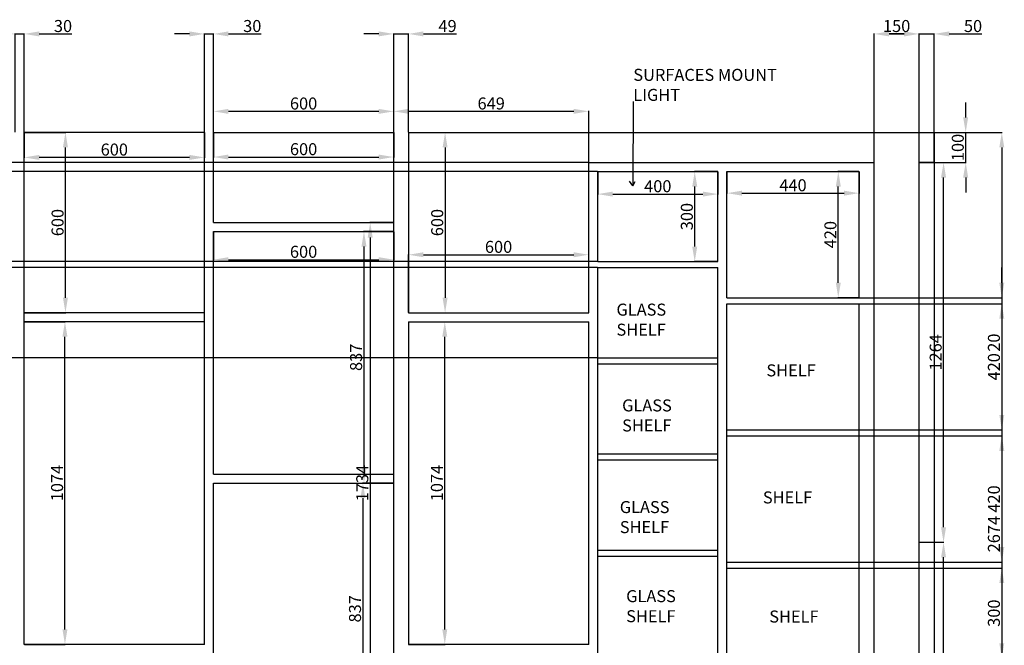
# Model space of a CAD drawing. Units: millimetres. Extents: x -2182 to 7969, y 257 to 4097.
# Tile 5 of 5: x 4692 to 7969, y 1457 to 3539. Entities that reach past the tile are written whole.
import ezdxf

# ---------------------------------------------------------------- set-up
doc = ezdxf.new("R2010")
doc.units = ezdxf.units.MM
for name, color, linetype, lineweight in [('A-ANNO-DIMS', 2, 'Continuous', 18), ('A-ANNO-TEXT', 3, 'Continuous', 18), ('A-ELEV', 7, 'Continuous', 25)]:
    doc.layers.add(name, color=color, linetype=linetype, lineweight=lineweight)
doc.styles.get("Standard").update_dxf_attribs({"font": 'arial.ttf'})
doc.dimstyles.new('ISO-25', dxfattribs={"dimtxt": 40, "dimasz": 50, "dimexe": 1.25, "dimexo": 0.625, "dimtad": 1, "dimtxsty": 'Standard', "dimcen": 2.5, "dimadec": 0, "dimazin": 0, "dimtfac": 1, "dimtmove": 0, "dimatfit": 3, "dimfxl": 1, "dimarcsym": 0})

# ---------------------------------------------------------------- blocks, each defined once
blk = doc.blocks.new('*D53')
at = {"layer": 'A-ANNO-DIMS', "color": 0, "lineweight": -2, "transparency": 16777216}
for p, q in [((7686.6, 1800), (7768.3, 1800)), ((7767.1, 650), (7767.1, 1750)), ((7536.6, 600), (7768.3, 600))]:
    blk.add_line(p, q, dxfattribs=at)
at = {"layer": 'A-ANNO-DIMS', "color": 0, "transparency": 16777216}
for points in [[(7758.7, 1750), (7775.4, 1750), (7767.1, 1800)], [(7758.7, 650), (7775.4, 650), (7767.1, 600)]]:
    blk.add_solid(points, dxfattribs=at)
at = {"layer": 'Defpoints', "color": 0, "transparency": 16777216}
for p in [(7685.9, 1800), (7767.1, 1800), (7535.9, 600)]:
    blk.add_point(p, dxfattribs=at)
at = {"layer": 'A-ANNO-DIMS', "color": 0, "transparency": 16777216, "insert": (7746, 1200), "char_height": 40, "attachment_point": 5, "rotation": 90}
blk.add_mtext('1200', dxfattribs=at)
blk = doc.blocks.new('*D50')
at = {"layer": 'A-ANNO-DIMS', "color": 0, "lineweight": -2, "transparency": 16777216}
for p, q in [((7686.6, 3064), (7768.3, 3064)), ((7767.1, 1850), (7767.1, 3014)), ((7686.6, 1800), (7768.3, 1800))]:
    blk.add_line(p, q, dxfattribs=at)
at = {"layer": 'A-ANNO-DIMS', "color": 0, "transparency": 16777216}
for points in [[(7758.7, 3014), (7775.4, 3014), (7767.1, 3064)], [(7758.7, 1850), (7775.4, 1850), (7767.1, 1800)]]:
    blk.add_solid(points, dxfattribs=at)
at = {"layer": 'Defpoints', "color": 0, "transparency": 16777216}
for p in [(7685.9, 3064), (7767.1, 3064), (7685.9, 1800)]:
    blk.add_point(p, dxfattribs=at)
at = {"layer": 'A-ANNO-DIMS', "color": 0, "transparency": 16777216, "insert": (7746, 2432), "char_height": 40, "attachment_point": 5, "rotation": 90}
blk.add_mtext('1264', dxfattribs=at)
blk = doc.blocks.new('*D51')
at = {"layer": 'A-ANNO-DIMS', "color": 0, "lineweight": -2, "transparency": 16777216}
for p, q in [((7840.7, 3214), (7840.7, 3264)), ((7736.6, 3164), (7841.9, 3164)), ((7840.7, 3064), (7840.7, 3164)), ((7737.8, 3064), (7841.9, 3064)), ((7840.7, 3014), (7840.7, 2964))]:
    blk.add_line(p, q, dxfattribs=at)
at = {"layer": 'A-ANNO-DIMS', "color": 0, "transparency": 16777216}
for points in [[(7832.3, 3214), (7849, 3214), (7840.7, 3164)], [(7832.3, 3014), (7849, 3014), (7840.7, 3064)]]:
    blk.add_solid(points, dxfattribs=at)
at = {"layer": 'Defpoints', "color": 0, "transparency": 16777216}
for p in [(7735.9, 3164), (7840.7, 3164), (7737.2, 3064)]:
    blk.add_point(p, dxfattribs=at)
at = {"layer": 'A-ANNO-DIMS', "color": 0, "transparency": 16777216, "insert": (7819.6, 3114), "char_height": 40, "attachment_point": 5, "rotation": 90}
blk.add_mtext('100', dxfattribs=at)
blk = doc.blocks.new('*D37')
at = {"layer": 'A-ANNO-DIMS', "color": 0, "lineweight": -2, "transparency": 16777216}
for p, q in [((5985.9, 2564.6), (5985.9, 2758.2)), ((6035.9, 2757), (6535.9, 2757)), ((6585.9, 2564.6), (6585.9, 2758.2))]:
    blk.add_line(p, q, dxfattribs=at)
at = {"layer": 'A-ANNO-DIMS', "color": 0, "transparency": 16777216}
for points in [[(6035.9, 2765.3), (6035.9, 2748.6), (5985.9, 2757)], [(6535.9, 2765.3), (6535.9, 2748.6), (6585.9, 2757)]]:
    blk.add_solid(points, dxfattribs=at)
at = {"layer": 'Defpoints', "color": 0, "transparency": 16777216}
for p in [(6585.9, 2757), (5985.9, 2564), (6585.9, 2564)]:
    blk.add_point(p, dxfattribs=at)
at = {"layer": 'A-ANNO-DIMS', "color": 0, "transparency": 16777216, "insert": (6285.9, 2778), "char_height": 40, "attachment_point": 5}
blk.add_mtext('600', dxfattribs=at)
blk = doc.blocks.new('*D38')
at = {"layer": 'A-ANNO-DIMS', "color": 0, "lineweight": -2, "transparency": 16777216}
for p, q in [((5986.6, 3164), (6109.1, 3164)), ((6107.9, 3114), (6107.9, 2614)), ((5986.6, 2564), (6109.1, 2564))]:
    blk.add_line(p, q, dxfattribs=at)
at = {"layer": 'A-ANNO-DIMS', "color": 0, "transparency": 16777216}
for points in [[(6099.5, 3114), (6116.2, 3114), (6107.9, 3164)], [(6099.5, 2614), (6116.2, 2614), (6107.9, 2564)]]:
    blk.add_solid(points, dxfattribs=at)
at = {"layer": 'Defpoints', "color": 0, "transparency": 16777216}
for p in [(5985.9, 3164), (5985.9, 2564), (6107.9, 2564)]:
    blk.add_point(p, dxfattribs=at)
at = {"layer": 'A-ANNO-DIMS', "color": 0, "transparency": 16777216, "insert": (6086.8, 2864), "char_height": 40, "attachment_point": 5, "rotation": 90}
blk.add_mtext('600', dxfattribs=at)
blk = doc.blocks.new('*D31')
at = {"layer": 'A-ANNO-DIMS', "color": 0, "lineweight": -2, "transparency": 16777216}
for p, q in [((5986.6, 2534), (6108.1, 2534)), ((6106.9, 1510), (6106.9, 2484)), ((5986.6, 1460), (6108.1, 1460))]:
    blk.add_line(p, q, dxfattribs=at)
at = {"layer": 'A-ANNO-DIMS', "color": 0, "transparency": 16777216}
for points in [[(6098.5, 2484), (6115.2, 2484), (6106.9, 2534)], [(6098.5, 1510), (6115.2, 1510), (6106.9, 1460)]]:
    blk.add_solid(points, dxfattribs=at)
at = {"layer": 'Defpoints', "color": 0, "transparency": 16777216}
for p in [(5985.9, 2534), (6106.9, 2534), (5985.9, 1460)]:
    blk.add_point(p, dxfattribs=at)
at = {"layer": 'A-ANNO-DIMS', "color": 0, "transparency": 16777216, "insert": (6085.8, 1997), "char_height": 40, "attachment_point": 5, "rotation": 90}
blk.add_mtext('1074', dxfattribs=at)
blk = doc.blocks.new('*D39')
at = {"layer": 'A-ANNO-DIMS', "color": 0, "lineweight": -2, "transparency": 16777216}
for p, q in [((5936.9, 3164.6), (5936.9, 3235.5)), ((6535.9, 3234.3), (5986.9, 3234.3)), ((6585.9, 3164.6), (6585.9, 3235.5))]:
    blk.add_line(p, q, dxfattribs=at)
at = {"layer": 'A-ANNO-DIMS', "color": 0, "transparency": 16777216}
for points in [[(5986.9, 3242.6), (5986.9, 3225.9), (5936.9, 3234.3)], [(6535.9, 3242.6), (6535.9, 3225.9), (6585.9, 3234.3)]]:
    blk.add_solid(points, dxfattribs=at)
at = {"layer": 'Defpoints', "color": 0, "transparency": 16777216}
for p in [(5936.9, 3234.3), (5936.9, 3164), (6585.9, 3164)]:
    blk.add_point(p, dxfattribs=at)
at = {"layer": 'A-ANNO-DIMS', "color": 0, "transparency": 16777216, "insert": (6261.4, 3255.3), "char_height": 40, "attachment_point": 5}
blk.add_mtext('649', dxfattribs=at)
blk = doc.blocks.new('*D40')
at = {"layer": 'A-ANNO-DIMS', "color": 0, "lineweight": -2, "transparency": 16777216}
for p, q in [((5936.3, 2864), (5857.3, 2864)), ((5858.6, 2814), (5858.6, 1180)), ((5936.3, 1130), (5857.3, 1130))]:
    blk.add_line(p, q, dxfattribs=at)
at = {"layer": 'A-ANNO-DIMS', "color": 0, "transparency": 16777216}
for points in [[(5850.2, 2814), (5866.9, 2814), (5858.6, 2864)], [(5850.2, 1180), (5866.9, 1180), (5858.6, 1130)]]:
    blk.add_solid(points, dxfattribs=at)
at = {"layer": 'Defpoints', "color": 0, "transparency": 16777216}
for p in [(5936.9, 2864), (5858.6, 1130), (5936.9, 1130)]:
    blk.add_point(p, dxfattribs=at)
at = {"layer": 'A-ANNO-DIMS', "color": 0, "transparency": 16777216, "insert": (5837.5, 1997), "char_height": 40, "attachment_point": 5, "rotation": 90}
blk.add_mtext('1734', dxfattribs=at)
blk = doc.blocks.new('*D41')
at = {"layer": 'A-ANNO-DIMS', "color": 0, "lineweight": -2, "transparency": 16777216}
for p, q in [((5336.9, 2833.4), (5336.9, 2739.3)), ((5936.9, 2833.4), (5936.9, 2739.3)), ((5386.9, 2740.5), (5886.9, 2740.5))]:
    blk.add_line(p, q, dxfattribs=at)
at = {"layer": 'A-ANNO-DIMS', "color": 0, "transparency": 16777216}
for points in [[(5386.9, 2748.8), (5386.9, 2732.2), (5336.9, 2740.5)], [(5886.9, 2748.8), (5886.9, 2732.2), (5936.9, 2740.5)]]:
    blk.add_solid(points, dxfattribs=at)
at = {"layer": 'Defpoints', "color": 0, "transparency": 16777216}
for p in [(5336.9, 2834), (5936.9, 2834), (5936.9, 2740.5)]:
    blk.add_point(p, dxfattribs=at)
at = {"layer": 'A-ANNO-DIMS', "color": 0, "transparency": 16777216, "insert": (5636.9, 2761.6), "char_height": 40, "attachment_point": 5}
blk.add_mtext('600', dxfattribs=at)
blk = doc.blocks.new('*D42')
at = {"layer": 'A-ANNO-DIMS', "color": 0, "lineweight": -2, "transparency": 16777216}
for p, q in [((5936.3, 2834), (5836.7, 2834)), ((5837.9, 2784), (5837.9, 2047)), ((5936.3, 1997), (5836.7, 1997))]:
    blk.add_line(p, q, dxfattribs=at)
at = {"layer": 'A-ANNO-DIMS', "color": 0, "transparency": 16777216}
for points in [[(5829.6, 2784), (5846.3, 2784), (5837.9, 2834)], [(5829.6, 2047), (5846.3, 2047), (5837.9, 1997)]]:
    blk.add_solid(points, dxfattribs=at)
at = {"layer": 'Defpoints', "color": 0, "transparency": 16777216}
for p in [(5936.9, 2834), (5837.9, 1997), (5936.9, 1997)]:
    blk.add_point(p, dxfattribs=at)
at = {"layer": 'A-ANNO-DIMS', "color": 0, "transparency": 16777216, "insert": (5816.9, 2415.5), "char_height": 40, "attachment_point": 5, "rotation": 90}
blk.add_mtext('837', dxfattribs=at)
blk = doc.blocks.new('*D43')
at = {"layer": 'A-ANNO-DIMS', "color": 0, "lineweight": -2, "transparency": 16777216}
for p, q in [((5336.9, 3163.4), (5336.9, 3080.9)), ((5936.9, 3163.4), (5936.9, 3080.9)), ((5386.9, 3082.2), (5886.9, 3082.2))]:
    blk.add_line(p, q, dxfattribs=at)
at = {"layer": 'A-ANNO-DIMS', "color": 0, "transparency": 16777216}
for points in [[(5386.9, 3090.5), (5386.9, 3073.9), (5336.9, 3082.2)], [(5886.9, 3090.5), (5886.9, 3073.9), (5936.9, 3082.2)]]:
    blk.add_solid(points, dxfattribs=at)
at = {"layer": 'Defpoints', "color": 0, "transparency": 16777216}
for p in [(5336.9, 3164), (5936.9, 3164), (5936.9, 3082.2)]:
    blk.add_point(p, dxfattribs=at)
at = {"layer": 'A-ANNO-DIMS', "color": 0, "transparency": 16777216, "insert": (5636.9, 3103.2), "char_height": 40, "attachment_point": 5}
blk.add_mtext('600', dxfattribs=at)
blk = doc.blocks.new('*D33')
at = {"layer": 'A-ANNO-DIMS', "color": 0, "lineweight": -2, "transparency": 16777216}
for p, q in [((5936.3, 1997), (5833.1, 1997)), ((5834.4, 1947), (5834.4, 1210)), ((5936.3, 1160), (5833.1, 1160))]:
    blk.add_line(p, q, dxfattribs=at)
at = {"layer": 'A-ANNO-DIMS', "color": 0, "transparency": 16777216}
for points in [[(5826, 1947), (5842.7, 1947), (5834.4, 1997)], [(5826, 1210), (5842.7, 1210), (5834.4, 1160)]]:
    blk.add_solid(points, dxfattribs=at)
at = {"layer": 'Defpoints', "color": 0, "transparency": 16777216}
for p in [(5936.9, 1997), (5834.4, 1160), (5936.9, 1160)]:
    blk.add_point(p, dxfattribs=at)
at = {"layer": 'A-ANNO-DIMS', "color": 0, "transparency": 16777216, "insert": (5813.3, 1578.5), "char_height": 40, "attachment_point": 5, "rotation": 90}
blk.add_mtext('837', dxfattribs=at)
blk = doc.blocks.new('*D45')
at = {"layer": 'A-ANNO-DIMS', "color": 0, "lineweight": -2, "transparency": 16777216}
for p, q in [((5336.9, 3164.6), (5336.9, 3235.4)), ((5886.9, 3234.2), (5386.9, 3234.2)), ((5936.9, 3164.6), (5936.9, 3235.4))]:
    blk.add_line(p, q, dxfattribs=at)
at = {"layer": 'A-ANNO-DIMS', "color": 0, "transparency": 16777216}
for points in [[(5386.9, 3242.5), (5386.9, 3225.8), (5336.9, 3234.2)], [(5886.9, 3242.5), (5886.9, 3225.8), (5936.9, 3234.2)]]:
    blk.add_solid(points, dxfattribs=at)
at = {"layer": 'Defpoints', "color": 0, "transparency": 16777216}
for p in [(5336.9, 3234.2), (5336.9, 3164), (5936.9, 3164)]:
    blk.add_point(p, dxfattribs=at)
at = {"layer": 'A-ANNO-DIMS', "color": 0, "transparency": 16777216, "insert": (5636.9, 3255.2), "char_height": 40, "attachment_point": 5}
blk.add_mtext('600', dxfattribs=at)
blk = doc.blocks.new('*D48')
at = {"layer": 'A-ANNO-DIMS', "color": 0, "lineweight": -2, "transparency": 16777216}
for p, q in [((4707.6, 2534), (4843.8, 2534)), ((4842.6, 1510), (4842.6, 2484)), ((4707.6, 1460), (4843.8, 1460))]:
    blk.add_line(p, q, dxfattribs=at)
at = {"layer": 'A-ANNO-DIMS', "color": 0, "transparency": 16777216}
for points in [[(4834.2, 2484), (4850.9, 2484), (4842.6, 2534)], [(4834.2, 1510), (4850.9, 1510), (4842.6, 1460)]]:
    blk.add_solid(points, dxfattribs=at)
at = {"layer": 'Defpoints', "color": 0, "transparency": 16777216}
for p in [(4706.9, 2534), (4842.6, 2534), (4706.9, 1460)]:
    blk.add_point(p, dxfattribs=at)
at = {"layer": 'A-ANNO-DIMS', "color": 0, "transparency": 16777216, "insert": (4821.5, 1997), "char_height": 40, "attachment_point": 5, "rotation": 90}
blk.add_mtext('1074', dxfattribs=at)
blk = doc.blocks.new('*D49')
at = {"layer": 'A-ANNO-DIMS', "color": 0, "lineweight": -2, "transparency": 16777216}
for p, q in [((4707.6, 3164), (4845.5, 3164)), ((4844.2, 2614), (4844.2, 3114)), ((4707.6, 2564), (4845.5, 2564))]:
    blk.add_line(p, q, dxfattribs=at)
at = {"layer": 'A-ANNO-DIMS', "color": 0, "transparency": 16777216}
for points in [[(4835.9, 3114), (4852.6, 3114), (4844.2, 3164)], [(4835.9, 2614), (4852.6, 2614), (4844.2, 2564)]]:
    blk.add_solid(points, dxfattribs=at)
at = {"layer": 'Defpoints', "color": 0, "transparency": 16777216}
for p in [(4706.9, 3164), (4844.2, 3164), (4706.9, 2564)]:
    blk.add_point(p, dxfattribs=at)
at = {"layer": 'A-ANNO-DIMS', "color": 0, "transparency": 16777216, "insert": (4823.2, 2864), "char_height": 40, "attachment_point": 5, "rotation": 90}
blk.add_mtext('600', dxfattribs=at)
blk = doc.blocks.new('*D46')
at = {"layer": 'A-ANNO-DIMS', "color": 0, "lineweight": -2, "transparency": 16777216}
for p, q in [((4706.9, 3163.4), (4706.9, 3079.6)), ((5306.9, 3163.4), (5306.9, 3079.6)), ((5256.9, 3080.9), (4756.9, 3080.9))]:
    blk.add_line(p, q, dxfattribs=at)
at = {"layer": 'A-ANNO-DIMS', "color": 0, "transparency": 16777216}
for points in [[(4756.9, 3089.2), (4756.9, 3072.5), (4706.9, 3080.9)], [(5256.9, 3089.2), (5256.9, 3072.5), (5306.9, 3080.9)]]:
    blk.add_solid(points, dxfattribs=at)
at = {"layer": 'Defpoints', "color": 0, "transparency": 16777216}
for p in [(4706.9, 3164), (5306.9, 3164), (4706.9, 3080.9)]:
    blk.add_point(p, dxfattribs=at)
at = {"layer": 'A-ANNO-DIMS', "color": 0, "transparency": 16777216, "insert": (5006.9, 3101.9), "char_height": 40, "attachment_point": 5}
blk.add_mtext('600', dxfattribs=at)
blk = doc.blocks.new('*D57')
at = {"layer": 'A-ANNO-DIMS', "color": 0, "lineweight": -2, "transparency": 16777216}
for p, q in [((7015.3, 3034), (6937.6, 3034)), ((6938.8, 2784), (6938.8, 2984)), ((7015.3, 2734), (6937.6, 2734))]:
    blk.add_line(p, q, dxfattribs=at)
at = {"layer": 'A-ANNO-DIMS', "color": 0, "transparency": 16777216}
for points in [[(6930.5, 2984), (6947.2, 2984), (6938.8, 3034)], [(6930.5, 2784), (6947.2, 2784), (6938.8, 2734)]]:
    blk.add_solid(points, dxfattribs=at)
at = {"layer": 'Defpoints', "color": 0, "transparency": 16777216}
for p in [(6938.8, 3034), (7015.9, 3034), (7015.9, 2734)]:
    blk.add_point(p, dxfattribs=at)
at = {"layer": 'A-ANNO-DIMS', "color": 0, "transparency": 16777216, "insert": (6917.8, 2884), "char_height": 40, "attachment_point": 5, "rotation": 90}
blk.add_mtext('300', dxfattribs=at)
blk = doc.blocks.new('*D58')
at = {"layer": 'A-ANNO-DIMS', "color": 0, "lineweight": -2, "transparency": 16777216}
for p, q in [((6615.9, 3033.4), (6615.9, 2957.6)), ((7015.9, 3033.4), (7015.9, 2957.6)), ((6665.9, 2958.8), (6965.9, 2958.8))]:
    blk.add_line(p, q, dxfattribs=at)
at = {"layer": 'A-ANNO-DIMS', "color": 0, "transparency": 16777216}
for points in [[(6665.9, 2967.2), (6665.9, 2950.5), (6615.9, 2958.8)], [(6965.9, 2967.2), (6965.9, 2950.5), (7015.9, 2958.8)]]:
    blk.add_solid(points, dxfattribs=at)
at = {"layer": 'Defpoints', "color": 0, "transparency": 16777216}
for p in [(6615.9, 3034), (7015.9, 3034), (7015.9, 2958.8)]:
    blk.add_point(p, dxfattribs=at)
at = {"layer": 'A-ANNO-DIMS', "color": 0, "transparency": 16777216, "insert": (6815.9, 2979.9), "char_height": 40, "attachment_point": 5}
blk.add_mtext('400', dxfattribs=at)
blk = doc.blocks.new('*D59')
at = {"layer": 'A-ANNO-DIMS', "color": 0, "lineweight": -2, "transparency": 16777216}
for p, q in [((7045.9, 3033.4), (7045.9, 2960.7)), ((7485.9, 3033.4), (7485.9, 2960.7)), ((7095.9, 2961.9), (7435.9, 2961.9))]:
    blk.add_line(p, q, dxfattribs=at)
at = {"layer": 'A-ANNO-DIMS', "color": 0, "transparency": 16777216}
for points in [[(7095.9, 2970.3), (7095.9, 2953.6), (7045.9, 2961.9)], [(7435.9, 2970.3), (7435.9, 2953.6), (7485.9, 2961.9)]]:
    blk.add_solid(points, dxfattribs=at)
at = {"layer": 'Defpoints', "color": 0, "transparency": 16777216}
for p in [(7045.9, 3034), (7485.9, 3034), (7485.9, 2961.9)]:
    blk.add_point(p, dxfattribs=at)
at = {"layer": 'A-ANNO-DIMS', "color": 0, "transparency": 16777216, "insert": (7265.9, 2983), "char_height": 40, "attachment_point": 5}
blk.add_mtext('440', dxfattribs=at)
blk = doc.blocks.new('*D60')
at = {"layer": 'A-ANNO-DIMS', "color": 0, "lineweight": -2, "transparency": 16777216}
for p, q in [((7485.3, 3034), (7415.5, 3034)), ((7416.7, 2664), (7416.7, 2984)), ((7485.3, 2614), (7415.5, 2614))]:
    blk.add_line(p, q, dxfattribs=at)
at = {"layer": 'A-ANNO-DIMS', "color": 0, "transparency": 16777216}
for points in [[(7408.4, 2984), (7425, 2984), (7416.7, 3034)], [(7408.4, 2664), (7425, 2664), (7416.7, 2614)]]:
    blk.add_solid(points, dxfattribs=at)
at = {"layer": 'Defpoints', "color": 0, "transparency": 16777216}
for p in [(7416.7, 3034), (7485.9, 3034), (7485.9, 2614)]:
    blk.add_point(p, dxfattribs=at)
at = {"layer": 'A-ANNO-DIMS', "color": 0, "transparency": 16777216, "insert": (7395.7, 2824), "char_height": 40, "attachment_point": 5, "rotation": 90}
blk.add_mtext('420', dxfattribs=at)
blk = doc.blocks.new('*D77')
at = {"layer": 'A-ANNO-DIMS', "color": 0, "lineweight": -2, "transparency": 16777216}
for p, q in [((7735.9, 3063.4), (7735.9, 263.7)), ((3426.9, 489.4), (3426.9, 263.7)), ((3476.9, 265), (7685.9, 265))]:
    blk.add_line(p, q, dxfattribs=at)
at = {"layer": 'A-ANNO-DIMS', "color": 0, "transparency": 16777216}
for points in [[(3476.9, 273.3), (3476.9, 256.7), (3426.9, 265)], [(7685.9, 273.3), (7685.9, 256.7), (7735.9, 265)]]:
    blk.add_solid(points, dxfattribs=at)
at = {"layer": 'Defpoints', "color": 0, "transparency": 16777216}
for p in [(7735.9, 3064), (3426.9, 490), (7735.9, 265)]:
    blk.add_point(p, dxfattribs=at)
at = {"layer": 'A-ANNO-DIMS', "color": 0, "transparency": 16777216, "insert": (5581.4, 286.1), "char_height": 40, "attachment_point": 5}
blk.add_mtext('4309', dxfattribs=at)
blk = doc.blocks.new('*D79')
at = {"layer": 'A-ANNO-DIMS', "color": 0, "lineweight": -2, "transparency": 16777216}
for p, q in [((7736.6, 3164), (7962.2, 3164)), ((7960.9, 3114), (7960.9, 540)), ((3427.6, 490), (7962.2, 490))]:
    blk.add_line(p, q, dxfattribs=at)
at = {"layer": 'A-ANNO-DIMS', "color": 0, "transparency": 16777216}
for points in [[(7952.6, 3114), (7969.3, 3114), (7960.9, 3164)], [(7952.6, 540), (7969.3, 540), (7960.9, 490)]]:
    blk.add_solid(points, dxfattribs=at)
at = {"layer": 'Defpoints', "color": 0, "transparency": 16777216}
for p in [(7735.9, 3164), (3426.9, 490), (7960.9, 490)]:
    blk.add_point(p, dxfattribs=at)
at = {"layer": 'A-ANNO-DIMS', "color": 0, "transparency": 16777216, "insert": (7939.9, 1827), "char_height": 40, "attachment_point": 5, "rotation": 90}
blk.add_mtext('2674', dxfattribs=at)
blk = doc.blocks.new('*D82')
at = {"layer": 'A-ANNO-DIMS', "color": 0, "lineweight": -2, "transparency": 16777216}
for p, q in [((4626.9, 3492), (4576.9, 3492)), ((4676.9, 3164.6), (4676.9, 3493.3)), ((4676.9, 3492), (4706.9, 3492)), ((4706.9, 3164.6), (4706.9, 3493.3)), ((4756.9, 3492), (4865.3, 3492))]:
    blk.add_line(p, q, dxfattribs=at)
at = {"layer": 'A-ANNO-DIMS', "color": 0, "transparency": 16777216}
for points in [[(4626.9, 3500.4), (4626.9, 3483.7), (4676.9, 3492)], [(4756.9, 3500.4), (4756.9, 3483.7), (4706.9, 3492)]]:
    blk.add_solid(points, dxfattribs=at)
at = {"layer": 'Defpoints', "color": 0, "transparency": 16777216}
for p in [(4706.9, 3492), (4676.9, 3164), (4706.9, 3164)]:
    blk.add_point(p, dxfattribs=at)
at = {"layer": 'A-ANNO-DIMS', "color": 0, "transparency": 16777216, "insert": (4836.1, 3513.1), "char_height": 40, "attachment_point": 5}
blk.add_mtext('30', dxfattribs=at)
blk = doc.blocks.new('*D83')
at = {"layer": 'A-ANNO-DIMS', "color": 0, "lineweight": -2, "transparency": 16777216}
for p, q in [((5256.9, 3492), (5206.9, 3492)), ((5306.9, 3164.6), (5306.9, 3493.3)), ((5306.9, 3492), (5336.9, 3492)), ((5336.9, 3164.6), (5336.9, 3493.3)), ((5386.9, 3492), (5495.3, 3492))]:
    blk.add_line(p, q, dxfattribs=at)
at = {"layer": 'A-ANNO-DIMS', "color": 0, "transparency": 16777216}
for points in [[(5256.9, 3500.4), (5256.9, 3483.7), (5306.9, 3492)], [(5386.9, 3500.4), (5386.9, 3483.7), (5336.9, 3492)]]:
    blk.add_solid(points, dxfattribs=at)
at = {"layer": 'Defpoints', "color": 0, "transparency": 16777216}
for p in [(5336.9, 3492), (5306.9, 3164), (5336.9, 3164)]:
    blk.add_point(p, dxfattribs=at)
at = {"layer": 'A-ANNO-DIMS', "color": 0, "transparency": 16777216, "insert": (5466.1, 3513.1), "char_height": 40, "attachment_point": 5}
blk.add_mtext('30', dxfattribs=at)
blk = doc.blocks.new('*D84')
at = {"layer": 'A-ANNO-DIMS', "color": 0, "lineweight": -2, "transparency": 16777216}
for p, q in [((5886.9, 3492), (5836.9, 3492)), ((5936.9, 3164.6), (5936.9, 3493.3)), ((5936.9, 3492), (5985.9, 3492)), ((5985.9, 3164.6), (5985.9, 3493.3)), ((6035.9, 3492), (6146.2, 3492))]:
    blk.add_line(p, q, dxfattribs=at)
at = {"layer": 'A-ANNO-DIMS', "color": 0, "transparency": 16777216}
for points in [[(5886.9, 3500.4), (5886.9, 3483.7), (5936.9, 3492)], [(6035.9, 3500.4), (6035.9, 3483.7), (5985.9, 3492)]]:
    blk.add_solid(points, dxfattribs=at)
at = {"layer": 'Defpoints', "color": 0, "transparency": 16777216}
for p in [(5985.9, 3492), (5936.9, 3164), (5985.9, 3164)]:
    blk.add_point(p, dxfattribs=at)
at = {"layer": 'A-ANNO-DIMS', "color": 0, "transparency": 16777216, "insert": (6116.1, 3513.1), "char_height": 40, "attachment_point": 5}
blk.add_mtext('49', dxfattribs=at)
blk = doc.blocks.new('*D88')
at = {"layer": 'A-ANNO-DIMS', "color": 0, "lineweight": -2, "transparency": 16777216}
for p, q in [((7535.9, 3064.6), (7535.9, 3493.3)), ((7585.9, 3492), (7635.9, 3492)), ((7685.9, 3064.6), (7685.9, 3493.3))]:
    blk.add_line(p, q, dxfattribs=at)
at = {"layer": 'A-ANNO-DIMS', "color": 0, "transparency": 16777216}
for points in [[(7585.9, 3500.4), (7585.9, 3483.7), (7535.9, 3492)], [(7635.9, 3500.4), (7635.9, 3483.7), (7685.9, 3492)]]:
    blk.add_solid(points, dxfattribs=at)
at = {"layer": 'Defpoints', "color": 0, "transparency": 16777216}
for p in [(7685.9, 3492), (7535.9, 3064), (7685.9, 3064)]:
    blk.add_point(p, dxfattribs=at)
at = {"layer": 'A-ANNO-DIMS', "color": 0, "transparency": 16777216, "insert": (7610.9, 3513.1), "char_height": 40, "attachment_point": 5}
blk.add_mtext('150', dxfattribs=at)
blk = doc.blocks.new('*D89')
at = {"layer": 'A-ANNO-DIMS', "color": 0, "lineweight": -2, "transparency": 16777216}
for p, q in [((7635.9, 3492), (7585.9, 3492)), ((7685.9, 3064.6), (7685.9, 3493.3)), ((7685.9, 3492), (7735.9, 3492)), ((7735.9, 3064.6), (7735.9, 3493.3)), ((7785.9, 3492), (7894.4, 3492))]:
    blk.add_line(p, q, dxfattribs=at)
at = {"layer": 'A-ANNO-DIMS', "color": 0, "transparency": 16777216}
for points in [[(7635.9, 3500.4), (7635.9, 3483.7), (7685.9, 3492)], [(7785.9, 3500.4), (7785.9, 3483.7), (7735.9, 3492)]]:
    blk.add_solid(points, dxfattribs=at)
at = {"layer": 'Defpoints', "color": 0, "transparency": 16777216}
for p in [(7735.9, 3492), (7685.9, 3064), (7735.9, 3064)]:
    blk.add_point(p, dxfattribs=at)
at = {"layer": 'A-ANNO-DIMS', "color": 0, "transparency": 16777216, "insert": (7865.2, 3513.1), "char_height": 40, "attachment_point": 5}
blk.add_mtext('50', dxfattribs=at)
blk = doc.blocks.new('*D92')
at = {"layer": 'A-ANNO-DIMS', "color": 0, "lineweight": -2, "transparency": 16777216}
for p, q in [((3201.9, 3114), (3201.9, 3164)), ((6585.3, 3064), (3200.7, 3064)), ((3201.9, 3064), (3201.9, 3034)), ((6615.3, 3034), (3200.7, 3034)), ((3201.9, 2984), (3201.9, 2875.6))]:
    blk.add_line(p, q, dxfattribs=at)
at = {"layer": 'A-ANNO-DIMS', "color": 0, "transparency": 16777216}
for points in [[(3193.6, 3114), (3210.3, 3114), (3201.9, 3064)], [(3193.6, 2984), (3210.3, 2984), (3201.9, 3034)]]:
    blk.add_solid(points, dxfattribs=at)
at = {"layer": 'Defpoints', "color": 0, "transparency": 16777216}
for p in [(6585.9, 3064), (3201.9, 3034), (6615.9, 3034)]:
    blk.add_point(p, dxfattribs=at)
at = {"layer": 'A-ANNO-DIMS', "color": 0, "transparency": 16777216, "insert": (3180.9, 2904.8), "char_height": 40, "attachment_point": 5, "rotation": 90}
blk.add_mtext('30', dxfattribs=at)
blk = doc.blocks.new('*D93')
at = {"layer": 'A-ANNO-DIMS', "color": 0, "lineweight": -2, "transparency": 16777216}
for p, q in [((3201.9, 2784), (3201.9, 2834)), ((6615.3, 2734), (3200.7, 2734)), ((3201.9, 2734), (3201.9, 2714)), ((6615.3, 2714), (3200.7, 2714)), ((3201.9, 2664), (3201.9, 2554.9))]:
    blk.add_line(p, q, dxfattribs=at)
at = {"layer": 'A-ANNO-DIMS', "color": 0, "transparency": 16777216}
for points in [[(3193.6, 2784), (3210.3, 2784), (3201.9, 2734)], [(3193.6, 2664), (3210.3, 2664), (3201.9, 2714)]]:
    blk.add_solid(points, dxfattribs=at)
at = {"layer": 'Defpoints', "color": 0, "transparency": 16777216}
for p in [(6615.9, 2734), (3201.9, 2714), (6615.9, 2714)]:
    blk.add_point(p, dxfattribs=at)
at = {"layer": 'A-ANNO-DIMS', "color": 0, "transparency": 16777216, "insert": (3180.9, 2584.4), "char_height": 40, "attachment_point": 5, "rotation": 90}
blk.add_mtext('20', dxfattribs=at)
blk = doc.blocks.new('*D94')
at = {"layer": 'A-ANNO-DIMS', "color": 0, "lineweight": -2, "transparency": 16777216}
for p, q in [((6615.3, 2714), (3200.7, 2714)), ((3201.9, 2664), (3201.9, 2464)), ((6615.3, 2414), (3200.7, 2414))]:
    blk.add_line(p, q, dxfattribs=at)
at = {"layer": 'A-ANNO-DIMS', "color": 0, "transparency": 16777216}
for points in [[(3193.6, 2664), (3210.3, 2664), (3201.9, 2714)], [(3193.6, 2464), (3210.3, 2464), (3201.9, 2414)]]:
    blk.add_solid(points, dxfattribs=at)
at = {"layer": 'Defpoints', "color": 0, "transparency": 16777216}
for p in [(6615.9, 2714), (3201.9, 2414), (6615.9, 2414)]:
    blk.add_point(p, dxfattribs=at)
at = {"layer": 'A-ANNO-DIMS', "color": 0, "transparency": 16777216, "insert": (3180.9, 2564), "char_height": 40, "attachment_point": 5, "rotation": 90}
blk.add_mtext('300', dxfattribs=at)
blk = doc.blocks.new('*D96')
at = {"layer": 'A-ANNO-DIMS', "color": 0, "lineweight": -2, "transparency": 16777216}
for p, q in [((7960.9, 2664), (7960.9, 2714)), ((7486.6, 2614), (7962.2, 2614)), ((7486.6, 2594), (7962.2, 2594)), ((7960.9, 2614), (7960.9, 2594)), ((7960.9, 2544), (7960.9, 2434.9))]:
    blk.add_line(p, q, dxfattribs=at)
at = {"layer": 'A-ANNO-DIMS', "color": 0, "transparency": 16777216}
for points in [[(7952.6, 2664), (7969.3, 2664), (7960.9, 2614)], [(7952.6, 2544), (7969.3, 2544), (7960.9, 2594)]]:
    blk.add_solid(points, dxfattribs=at)
at = {"layer": 'Defpoints', "color": 0, "transparency": 16777216}
for p in [(7485.9, 2614), (7485.9, 2594), (7960.9, 2594)]:
    blk.add_point(p, dxfattribs=at)
at = {"layer": 'A-ANNO-DIMS', "color": 0, "transparency": 16777216, "insert": (7939.9, 2464.4), "char_height": 40, "attachment_point": 5, "rotation": 90}
blk.add_mtext('20', dxfattribs=at)
blk = doc.blocks.new('*D97')
at = {"layer": 'A-ANNO-DIMS', "color": 0, "lineweight": -2, "transparency": 16777216}
for p, q in [((7486.6, 2594), (7962.2, 2594)), ((7960.9, 2544), (7960.9, 2224)), ((7486.6, 2174), (7962.2, 2174))]:
    blk.add_line(p, q, dxfattribs=at)
at = {"layer": 'A-ANNO-DIMS', "color": 0, "transparency": 16777216}
for points in [[(7952.6, 2544), (7969.3, 2544), (7960.9, 2594)], [(7952.6, 2224), (7969.3, 2224), (7960.9, 2174)]]:
    blk.add_solid(points, dxfattribs=at)
at = {"layer": 'Defpoints', "color": 0, "transparency": 16777216}
for p in [(7485.9, 2594), (7485.9, 2174), (7960.9, 2174)]:
    blk.add_point(p, dxfattribs=at)
at = {"layer": 'A-ANNO-DIMS', "color": 0, "transparency": 16777216, "insert": (7939.9, 2384), "char_height": 40, "attachment_point": 5, "rotation": 90}
blk.add_mtext('420', dxfattribs=at)
blk = doc.blocks.new('*D98')
at = {"layer": 'A-ANNO-DIMS', "color": 0, "lineweight": -2, "transparency": 16777216}
for p, q in [((7486.6, 2154), (7962.2, 2154)), ((7960.9, 2104), (7960.9, 1784)), ((7486.6, 1734), (7962.2, 1734))]:
    blk.add_line(p, q, dxfattribs=at)
at = {"layer": 'A-ANNO-DIMS', "color": 0, "transparency": 16777216}
for points in [[(7952.6, 2104), (7969.3, 2104), (7960.9, 2154)], [(7952.6, 1784), (7969.3, 1784), (7960.9, 1734)]]:
    blk.add_solid(points, dxfattribs=at)
at = {"layer": 'Defpoints', "color": 0, "transparency": 16777216}
for p in [(7485.9, 2154), (7485.9, 1734), (7960.9, 1734)]:
    blk.add_point(p, dxfattribs=at)
at = {"layer": 'A-ANNO-DIMS', "color": 0, "transparency": 16777216, "insert": (7939.9, 1944), "char_height": 40, "attachment_point": 5, "rotation": 90}
blk.add_mtext('420', dxfattribs=at)
blk = doc.blocks.new('*D99')
at = {"layer": 'A-ANNO-DIMS', "color": 0, "lineweight": -2, "transparency": 16777216}
for p, q in [((7486.6, 1714), (7962.2, 1714)), ((7960.9, 1664), (7960.9, 1464)), ((7486.6, 1414), (7962.2, 1414))]:
    blk.add_line(p, q, dxfattribs=at)
at = {"layer": 'A-ANNO-DIMS', "color": 0, "transparency": 16777216}
for points in [[(7952.6, 1664), (7969.3, 1664), (7960.9, 1714)], [(7952.6, 1464), (7969.3, 1464), (7960.9, 1414)]]:
    blk.add_solid(points, dxfattribs=at)
at = {"layer": 'Defpoints', "color": 0, "transparency": 16777216}
for p in [(7485.9, 1714), (7485.9, 1414), (7960.9, 1414)]:
    blk.add_point(p, dxfattribs=at)
at = {"layer": 'A-ANNO-DIMS', "color": 0, "transparency": 16777216, "insert": (7939.9, 1564), "char_height": 40, "attachment_point": 5, "rotation": 90}
blk.add_mtext('300', dxfattribs=at)

msp = doc.modelspace()

# ---------------------------------------------------------------- linework, layer by layer
at = {"layer": 'A-ELEV'}
for p, q in [((6734.4235, 3267.0268), (6733.3136, 2986.6436)), ((4706.9478, 1459.9911), (4706.9478, 3163.9911)), ((5306.9478, 3163.9911), (4706.9478, 3163.9911)), ((5306.9478, 1459.9911), (5306.9478, 3163.9911)), ((5336.9478, 2863.9911), (5336.9478, 3163.9911)), ((5336.9478, 3163.9911), (5936.9478, 3163.9911)), ((5936.9478, 1159.9911), (5936.9478, 3163.9911)), ((5985.9478, 3163.9911), (7735.9478, 3163.9911)), ((5985.9478, 3163.9911), (5985.9478, 2563.9911)), ((6585.9478, 2563.9911), (6585.9478, 3163.9911)), ((7735.9478, 3163.9911), (7735.9478, 3063.9911)), ((6585.9478, 3063.9911), (7535.9478, 3063.9911)), ((7535.9478, 599.9911), (7535.9478, 3063.9911)), ((7685.9478, 599.9911), (7685.9478, 3063.9911)), ((7735.9478, 3063.9911), (7685.9478, 3063.9911)), ((6615.9478, 3033.9911), (7015.9478, 3033.9911)), ((6615.9478, 2733.9911), (6615.9478, 3033.9911)), ((7015.9478, 2733.9911), (7015.9478, 3033.9911)), ((7045.9478, 3033.9911), (7485.9478, 3033.9911)), ((7045.9478, 2613.9911), (7045.9478, 3033.9911)), ((7485.9478, 2613.9911), (7485.9478, 3033.9911)), ((6733.3136, 2986.6436), (6721.4552, 3001.6567)), ((6733.3136, 2986.6436), (6740.8243, 3001.2796)), ((5336.9478, 2863.9911), (5936.9478, 2863.9911)), ((5336.9478, 2026.9911), (5336.9478, 2833.9911)), ((5336.9478, 2833.9911), (5936.9478, 2833.9911)), ((6615.9478, 2733.9911), (7015.9478, 2733.9911)), ((6615.9478, 489.9911), (6615.9478, 2713.9911)), ((6615.9478, 2713.9911), (7015.9478, 2713.9911)), ((7015.9478, 489.9911), (7015.9478, 2713.9911)), ((7045.9478, 2613.9911), (7485.9478, 2613.9911)), ((7045.9478, 489.9911), (7045.9478, 2593.9911)), ((7045.9478, 2593.9911), (7485.9478, 2593.9911)), ((7485.9478, 599.9911), (7485.9478, 2593.9911)), ((5306.9478, 2563.9911), (4706.9478, 2563.9911)), ((5985.9478, 2563.9911), (6585.9478, 2563.9911)), ((5306.9478, 2533.9911), (4706.9478, 2533.9911)), ((5985.9478, 2533.9911), (6585.9478, 2533.9911)), ((5985.9478, 2533.9911), (5985.9478, 1459.9911)), ((6585.9478, 1459.9911), (6585.9478, 2533.9911)), ((6615.9478, 2413.9911), (7015.9478, 2413.9911)), ((6615.9478, 2393.9911), (7015.9478, 2393.9911)), ((7045.9478, 2173.9911), (7485.9478, 2173.9911)), ((7045.9478, 2153.9911), (7485.9478, 2153.9911)), ((6615.9478, 2093.9911), (7015.9478, 2093.9911)), ((6615.9478, 2093.9911), (7015.9478, 2093.9911)), ((6615.9478, 2073.9911), (7015.9478, 2073.9911)), ((6615.9478, 2073.9911), (7015.9478, 2073.9911)), ((5336.9478, 2026.9911), (5936.9478, 2026.9911)), ((5336.9478, 1159.9911), (5336.9478, 1996.9911)), ((5336.9478, 1996.9911), (5936.9478, 1996.9911)), ((6615.9478, 1773.9911), (7015.9478, 1773.9911)), ((6615.9478, 1773.9911), (7015.9478, 1773.9911)), ((6615.9478, 1753.9911), (7015.9478, 1753.9911)), ((6615.9478, 1753.9911), (7015.9478, 1753.9911)), ((7045.9478, 1733.9911), (7485.9478, 1733.9911)), ((7045.9478, 1713.9911), (7485.9478, 1713.9911)), ((5306.9478, 1459.9911), (4706.9478, 1459.9911)), ((6585.9478, 1459.9911), (5985.9478, 1459.9911))]:
    msp.add_line(p, q, dxfattribs=at)

# ---------------------------------------------------------------- texts
at = {"layer": 'A-ANNO-TEXT', "char_height": 40, "attachment_point": 1}
for s, insert, width in [('SURFACES MOUNT\\P LIGHT', (6734.4235, 3375.7671), 716.323819), ('GLASS \\PSHELF', (6678.3624, 2594.2379), 482.986246), ('\\PSHELF', (7177.4018, 2458.7646), 482.986246), ('GLASS \\PSHELF', (6697.1168, 2275.4453), 482.986246), ('\\PSHELF', (7165.6258, 2035.865), 482.986246), ('GLASS \\PSHELF', (6689.4241, 1937.1162), 482.986246), ('GLASS \\PSHELF', (6710.6219, 1640.6166), 482.986246), ('\\PSHELF', (7186.9129, 1639.3946), 482.986246)]:
    msp.add_mtext(s, dxfattribs=dict(at, insert=insert, width=width))

# ---------------------------------------------------------------- dimensions: what is measured, and where the dimension line sits
at = {"layer": 'A-ANNO-DIMS'}
for base, p1, p2, override, picture, middle in [((4706.9478, 3492.0268), (4676.9478, 3163.9911), (4706.9478, 3163.9911), {"dimdec": 0, "dimlfac": 1, "dimrnd": 0, "dimzin": 0, "dimdsep": 46, "dimlunit": 2}, '*D82', (4836.1403, 3513.0883)), ((5336.9478, 3492.0268), (5306.9478, 3163.9911), (5336.9478, 3163.9911), {"dimdec": 0, "dimlfac": 1, "dimrnd": 0, "dimzin": 0, "dimdsep": 46, "dimlunit": 2}, '*D83', (5466.1403, 3513.0883)), ((5985.9478, 3492.0268), (5936.9478, 3163.9911), (5985.9478, 3163.9911), {"dimdec": 0, "dimlfac": 1, "dimrnd": 0, "dimzin": 0, "dimdsep": 46, "dimlunit": 2}, '*D84', (6116.068, 3513.0747)), ((7685.9478, 3492.0268), (7535.9478, 3063.9911), (7685.9478, 3063.9911), {"dimdec": 0, "dimlfac": 1, "dimrnd": 0, "dimzin": 0, "dimdsep": 46, "dimlunit": 2}, '*D88', (7610.9478, 3513.0747)), ((7735.9478, 3492.0268), (7685.9478, 3063.9911), (7735.9478, 3063.9911), {"dimdec": 0, "dimlfac": 1, "dimrnd": 0, "dimzin": 0, "dimdsep": 46, "dimlunit": 2}, '*D89', (7865.154, 3513.0747)), ((5336.9478, 3234.1574), (5936.9478, 3163.9911), (5336.9478, 3163.9911), {"dimclrd": 0, "dimclre": 0, "dimclrt": 0}, '*D45', (5636.9478, 3255.2053)), ((5936.9478, 3234.2728), (6585.9478, 3163.9911), (5936.9478, 3163.9911), {"dimclrd": 0, "dimclre": 0, "dimclrt": 0}, '*D39', (6261.4478, 3255.3207)), ((4706.9478, 3080.8621), (5306.9478, 3163.9911), (4706.9478, 3163.9911), {"dimclrd": 0, "dimclre": 0, "dimclrt": 0}, '*D46', (5006.9478, 3101.91)), ((5936.9478, 3082.1966), (5336.9478, 3163.9911), (5936.9478, 3163.9911), {"dimclrd": 0, "dimclre": 0, "dimclrt": 0}, '*D43', (5636.9478, 3103.2445)), ((7735.9478, 264.9911), (3426.9478, 489.9911), (7735.9478, 3063.9911), {"dimdec": 0, "dimlfac": 1, "dimrnd": 0, "dimzin": 0, "dimdsep": 46, "dimlunit": 2}, '*D77', (5581.4478, 286.0526)), ((7015.9478, 2958.8406), (6615.9478, 3033.9911), (7015.9478, 3033.9911), {"dimclrd": 0, "dimclre": 0, "dimclrt": 0}, '*D58', (6815.9478, 2979.8885)), ((7485.9478, 2961.9389), (7045.9478, 3033.9911), (7485.9478, 3033.9911), {"dimclrd": 0, "dimclre": 0, "dimclrt": 0}, '*D59', (7265.9478, 2982.9868)), ((5936.9478, 2740.5163), (5336.9478, 2833.9911), (5936.9478, 2833.9911), {"dimclrd": 0, "dimclre": 0, "dimclrt": 0}, '*D41', (5636.9478, 2761.5643)), ((6585.9478, 2756.9651), (5985.9478, 2563.9911), (6585.9478, 2563.9911), {"dimclrd": 0, "dimclre": 0, "dimclrt": 0}, '*D37', (6285.9478, 2778.013))]:
    dim = msp.add_linear_dim(base=base, p1=p1, p2=p2, dimstyle='ISO-25', override=override, dxfattribs=at)
    dim.commit()
    dim.dimension.update_dxf_attribs({"geometry": picture, "text_midpoint": middle})
for base, p1, p2, picture, middle in [((7840.6516, 3163.9911), (7737.1978, 3063.9911), (7735.9478, 3163.9911), '*D51', (7840.6516, 3113.9911)), ((4844.2396, 3163.9911), (4706.9478, 2563.9911), (4706.9478, 3163.9911), '*D49', (4844.2396, 2863.9911))]:
    dim = msp.add_linear_dim(base=base, p1=p1, p2=p2, angle=90, dimstyle='ISO-25', override={"dimclrd": 0, "dimclre": 0, "dimclrt": 0}, dxfattribs=at)
    dim.commit()
    dim.dimension.update_dxf_attribs({"geometry": picture, "text_midpoint": middle, "dimtype": 160})
for base, p1, p2, override, picture, middle in [((3201.9478, 3033.9911), (6585.9478, 3063.9911), (6615.9478, 3033.9911), {"dimdec": 0, "dimlfac": 1, "dimrnd": 0, "dimzin": 0, "dimdsep": 46, "dimlunit": 2}, '*D92', (3180.8862, 2904.7985)), ((7960.9478, 489.9911), (7735.9478, 3163.9911), (3426.9478, 489.9911), {"dimdec": 0, "dimlfac": 1, "dimrnd": 0, "dimzin": 0, "dimdsep": 46, "dimlunit": 2}, '*D79', (7939.8999, 1826.9911)), ((6107.8795, 2563.9911), (5985.9478, 3163.9911), (5985.9478, 2563.9911), {"dimclrd": 0, "dimclre": 0, "dimclrt": 0}, '*D38', (6086.8315, 2863.9911)), ((7767.0748, 3063.9911), (7685.9478, 1799.9911), (7685.9478, 3063.9911), {"dimasz": 50, "dimclrd": 0, "dimclre": 0, "dimclrt": 0}, '*D50', (7746.0269, 2431.9911)), ((6938.8236, 3033.9911), (7015.9478, 2733.9911), (7015.9478, 3033.9911), {"dimclrd": 0, "dimclre": 0, "dimclrt": 0}, '*D57', (6917.762, 2883.9911)), ((7416.7012, 3033.9911), (7485.9478, 2613.9911), (7485.9478, 3033.9911), {"dimclrd": 0, "dimclre": 0, "dimclrt": 0}, '*D60', (7395.6533, 2823.9911)), ((5858.5641, 1129.9911), (5936.9478, 2863.9911), (5936.9478, 1129.9911), {"dimclrd": 0, "dimclre": 0, "dimclrt": 0}, '*D40', (5837.5025, 1996.9911)), ((3201.9478, 2713.9911), (6615.9478, 2733.9911), (6615.9478, 2713.9911), {"dimdec": 0, "dimlfac": 1, "dimrnd": 0, "dimzin": 0, "dimdsep": 46, "dimlunit": 2}, '*D93', (3180.8999, 2584.4438)), ((5837.9295, 1996.9911), (5936.9478, 2833.9911), (5936.9478, 1996.9911), {"dimclrd": 0, "dimclre": 0, "dimclrt": 0}, '*D42', (5816.8679, 2415.4911)), ((3201.9478, 2413.9911), (6615.9478, 2713.9911), (6615.9478, 2413.9911), {"dimdec": 0, "dimlfac": 1, "dimrnd": 0, "dimzin": 0, "dimdsep": 46, "dimlunit": 2}, '*D94', (3180.8862, 2563.9911)), ((7960.9478, 2593.9911), (7485.9478, 2613.9911), (7485.9478, 2593.9911), {"dimdec": 0, "dimlfac": 1, "dimrnd": 0, "dimzin": 0, "dimdsep": 46, "dimlunit": 2}, '*D96', (7939.8999, 2464.4438)), ((7960.9478, 2173.9911), (7485.9478, 2593.9911), (7485.9478, 2173.9911), {"dimdec": 0, "dimlfac": 1, "dimrnd": 0, "dimzin": 0, "dimdsep": 46, "dimlunit": 2}, '*D97', (7939.8999, 2383.9911)), ((4842.5689, 2533.9911), (4706.9478, 1459.9911), (4706.9478, 2533.9911), {"dimclrd": 0, "dimclre": 0, "dimclrt": 0}, '*D48', (4821.521, 1996.9911)), ((6106.8561, 2533.9911), (5985.9478, 1459.9911), (5985.9478, 2533.9911), {"dimclrd": 0, "dimclre": 0, "dimclrt": 0}, '*D31', (6085.8081, 1996.9911)), ((7960.9478, 1733.9911), (7485.9478, 2153.9911), (7485.9478, 1733.9911), {"dimdec": 0, "dimlfac": 1, "dimrnd": 0, "dimzin": 0, "dimdsep": 46, "dimlunit": 2}, '*D98', (7939.8999, 1943.9911)), ((5834.375, 1159.9911), (5936.9478, 1996.9911), (5936.9478, 1159.9911), {"dimclrd": 0, "dimclre": 0, "dimclrt": 0}, '*D33', (5813.3135, 1578.4911)), ((7767.0748, 1799.9911), (7535.9478, 599.9911), (7685.9478, 1799.9911), {"dimclrd": 0, "dimclre": 0, "dimclrt": 0}, '*D53', (7746.0269, 1199.9911)), ((7960.9478, 1413.9911), (7485.9478, 1713.9911), (7485.9478, 1413.9911), {"dimdec": 0, "dimlfac": 1, "dimrnd": 0, "dimzin": 0, "dimdsep": 46, "dimlunit": 2}, '*D99', (7939.8862, 1563.9911))]:
    dim = msp.add_linear_dim(base=base, p1=p1, p2=p2, angle=90, dimstyle='ISO-25', override=override, dxfattribs=at)
    dim.commit()
    dim.dimension.update_dxf_attribs({"geometry": picture, "text_midpoint": middle})

doc.saveas('drawing.dxf')
